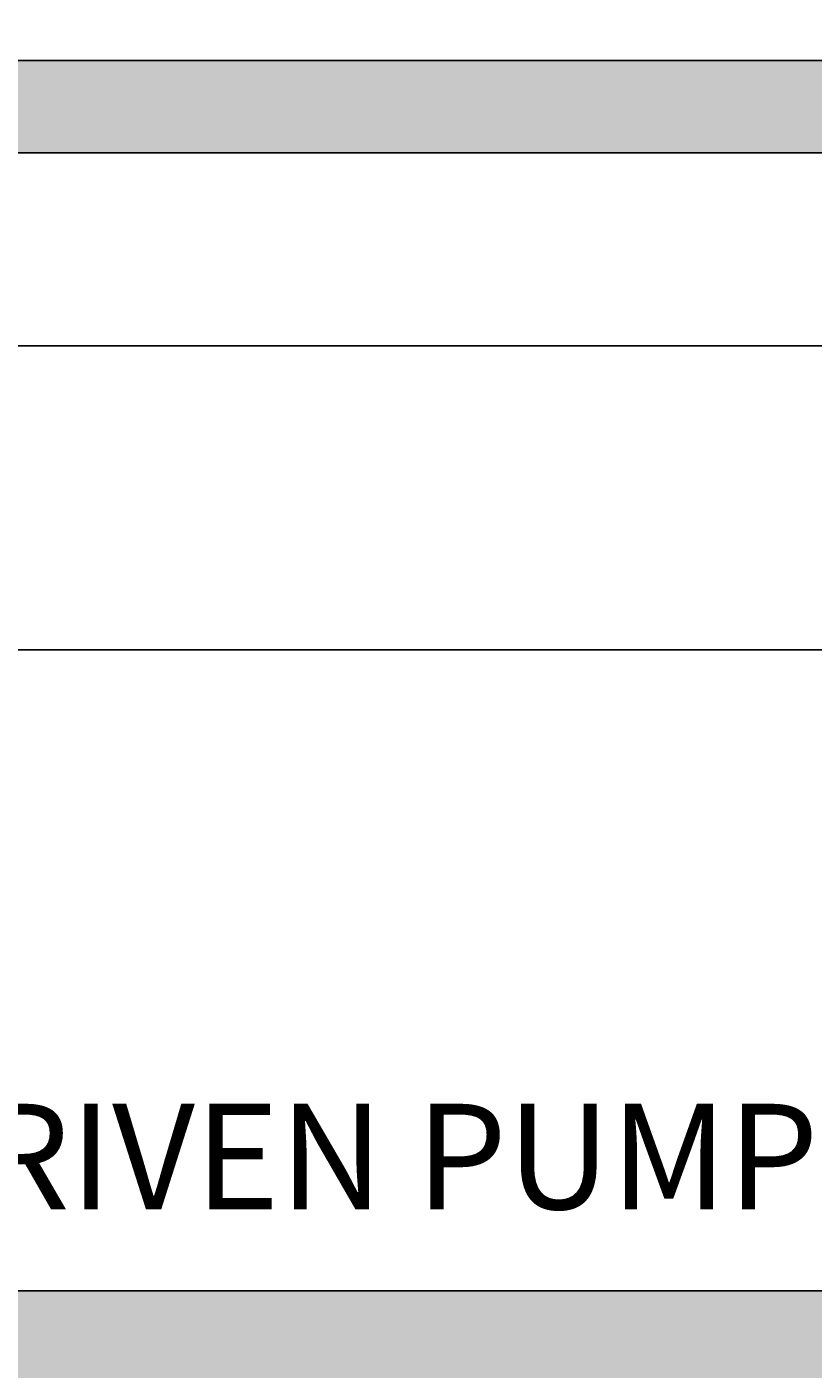
# Model space of a CAD drawing. Units: millimetres. Extents: x -11 to 280, y -4 to 208.
# Tile 43 of 55: x 121 to 151, y 106 to 157. Entities that reach past the tile are written whole.
import ezdxf

# ---------------------------------------------------------------- set-up
doc = ezdxf.new("R2010")
doc.units = ezdxf.units.MM
for name, color, linetype, lineweight in [('M-ANNO-TEXT', 7, 'Continuous', 18), ('M-DIMS', 2, 'Continuous', 18), ('M-HYDR-PRES', 7, 'Continuous', 25), ('M-HYDR-SUCT', 7, 'Continuous', 25)]:
    doc.layers.add(name, color=color, linetype=linetype, lineweight=lineweight)
doc.layers.add('M-HYDR-PRES-PATT', color=240, linetype='Continuous', lineweight=13, true_color=0xed1f24)
doc.layers.add('M-HYDR-SUCT-PATT', color=221, linetype='Continuous', lineweight=13, true_color=0xff7fdf)
doc.styles.get("Standard").update_dxf_attribs({"font": 'arial.ttf'})
doc.dimstyles.get("Standard").update_dxf_attribs({"dimtxt": 0.18, "dimasz": 0.18, "dimexe": 0.18, "dimexo": 0.0625, "dimgap": 0.09, "dimtad": 0, "dimtih": 1, "dimtoh": 1, "dimdec": 4, "dimzin": 0, "dimdsep": 46, "dimtxsty": 'Standard', "dimcen": 0.09, "dimadec": 0, "dimazin": 0, "dimtfac": 1, "dimtdec": 4, "dimtofl": 0, "dimtmove": 0, "dimatfit": 3, "dimfxl": 1, "dimtolj": 1, "dimtzin": 0, "dimarcsym": 0})

# ---------------------------------------------------------------- blocks, each defined once
blk = doc.blocks.new('*D5')
at = {"layer": 'Defpoints', "color": 0, "transparency": 16777216}
for p in [(24.759, 192.645), (-10.087, 11.435), (261.686, 11.435)]:
    blk.add_point(p, dxfattribs=at)
at = {"layer": 'M-DIMS', "color": 0, "lineweight": -2, "transparency": 16777216}
for p, q in [((24.696, 192.645), (-10.267, 192.645)), ((-10.087, 192.465), (-10.087, 102.222)), ((-10.087, 11.615), (-10.087, 101.858)), ((261.624, 11.435), (-10.267, 11.435))]:
    blk.add_line(p, q, dxfattribs=at)
at = {"layer": 'M-DIMS', "color": 0, "transparency": 16777216}
for points in [[(-10.117, 192.465), (-10.057, 192.465), (-10.087, 192.645)], [(-10.117, 11.615), (-10.057, 11.615), (-10.087, 11.435)]]:
    blk.add_solid(points, dxfattribs=at)
at = {"layer": 'M-DIMS', "color": 0, "transparency": 16777216, "insert": (-10.087, 102.04), "char_height": 0.18, "attachment_point": 5}
blk.add_mtext('\\A1;181.2', dxfattribs=at)
blk = doc.blocks.new('*D12')
at = {"layer": 'Defpoints', "color": 0, "transparency": 16777216}
for p in [(173.804, 207.495), (118.514, 96.485), (173.804, 89.387)]:
    blk.add_point(p, dxfattribs=at)
at = {"layer": 'M-DIMS', "color": 0, "lineweight": -2, "transparency": 16777216}
for p, q in [((118.514, 96.547), (118.514, 207.675)), ((118.694, 207.495), (145.765, 207.495)), ((173.624, 207.495), (146.553, 207.495)), ((173.804, 89.45), (173.804, 207.675))]:
    blk.add_line(p, q, dxfattribs=at)
at = {"layer": 'M-DIMS', "color": 0, "transparency": 16777216}
for points in [[(118.694, 207.525), (118.694, 207.465), (118.514, 207.495)], [(173.624, 207.525), (173.624, 207.465), (173.804, 207.495)]]:
    blk.add_solid(points, dxfattribs=at)
at = {"layer": 'M-DIMS', "color": 0, "transparency": 16777216, "insert": (146.159, 207.495), "char_height": 0.18, "attachment_point": 5}
blk.add_mtext('\\A1;55.29', dxfattribs=at)
blk = doc.blocks.new('*D14')
at = {"layer": 'Defpoints', "color": 0, "transparency": 16777216}
for p in [(-10.087, 144.661), (205.531, 144.661), (226.511, 133.123)]:
    blk.add_point(p, dxfattribs=at)
at = {"layer": 'M-DIMS', "color": 0, "lineweight": -2, "transparency": 16777216}
for p, q in [((205.469, 144.661), (-10.267, 144.661)), ((-10.087, 144.481), (-10.087, 139.074)), ((-10.087, 133.303), (-10.087, 138.71)), ((226.448, 133.123), (-10.267, 133.123))]:
    blk.add_line(p, q, dxfattribs=at)
at = {"layer": 'M-DIMS', "color": 0, "transparency": 16777216}
for points in [[(-10.117, 144.481), (-10.057, 144.481), (-10.087, 144.661)], [(-10.117, 133.303), (-10.057, 133.303), (-10.087, 133.123)]]:
    blk.add_solid(points, dxfattribs=at)
at = {"layer": 'M-DIMS', "color": 0, "transparency": 16777216, "insert": (-10.087, 138.892), "char_height": 0.18, "attachment_point": 5}
blk.add_mtext('\\A1;11.538', dxfattribs=at)

msp = doc.modelspace()

# ---------------------------------------------------------------- hatches: boundary and pattern name
at = {"layer": 'M-HYDR-PRES-PATT'}
h = msp.add_hatch(color=256, dxfattribs=at)
h.set_gradient(color1=(237, 31, 36), color2=(237, 31, 36), tint=1)
h.paths.add_polyline_path([(232.2, 133.1228), (228.7, 133.1228), (228.7, 108.8141), (102.7646, 108.8141), (102.7646, 105.3141), (232.2, 105.3141)])
h.paths.add_polyline_path([(128.8433, 105.3141), (125.3433, 105.3141), (125.3433, 91.7099, 1), (128.8433, 91.7099)])
h.paths.add_polyline_path([(229.1617, 78.7098), (196.7745, 78.7098, -0.4142136), (191.7745, 83.7098), (191.7745, 105.3141), (188.2745, 105.3141), (188.2745, 80.2098, 0.4142136), (193.2745, 75.2098), (225.6617, 75.2098), (225.6617, 43.5991), (229.1617, 43.5991)])
h.paths.add_polyline_path([(102.7646, 110.3704), (95.5776, 110.3704), (95.5776, 103.9022), (102.7646, 103.9022)])
h.paths.add_polyline_path([(100.7059, 107.2502), (99.1711, 106.3641), (99.1711, 106.8641), (97.1711, 106.8641), (97.1711, 107.6363), (99.1711, 107.6363), (99.1711, 108.1363)], flags=16)
h.paths.add_polyline_path([(234.6119, 138.4081), (226.5106, 138.4081), (226.5106, 133.1228), (234.6119, 133.1228)])
h.paths.add_polyline_path([(231.1963, 135.7055), (230.2965, 134.1786), (229.4241, 135.7213), (229.9241, 135.7168), (229.9418, 137.7167), (230.7141, 137.7099), (230.6963, 135.71)], flags=16)
at = {"layer": 'M-HYDR-SUCT-PATT'}
h = msp.add_hatch(color=256, dxfattribs=at)
h.set_gradient(color1=(255, 127, 223), color2=(255, 127, 223), tint=1, name='INVCYLINDER')
h.paths.add_polyline_path([(91.3629, 155.4768), (91.3629, 132.4768), (58.3629, 132.4768), (58.3629, 153.9768), (54.8629, 153.9768), (54.8629, 128.9768), (94.8629, 128.9768), (94.8629, 151.9768), (205.5315, 151.9768), (205.5315, 155.4768)])
h.paths.add_polyline_path([(91.3, 114.9452, 1), (78.8273, 114.9452), (78.8273, 108.8141), (42.6453, 108.8141), (42.6453, 153.9768), (39.1453, 153.9768), (39.1453, 105.3141), (78.8273, 105.3141), (78.8273, 98.1491, 1), (91.3, 98.1491), (91.3, 105.3141), (95.5776, 105.3141), (95.5776, 108.8141), (91.3, 108.8141)])
h.paths.add_polyline_path([(228.7, 138.4081), (232.2, 138.4081), (232.2, 144.6609), (228.7, 144.6609)])
h.paths.add_polyline_path([(253.1005, 151.9768, 1), (253.1005, 155.4768), (252.6001, 155.4768), (253.5249, 153.991, -0.1401047), (253.6005, 153.7268, -0.7542249), (252.676, 153.4626), (251.4221, 155.4768), (236.9353, 155.4768), (236.9353, 151.9768)])
h.paths.add_polyline_path([(30.8182, 40.7626), (30.8182, 36.7626), (60.8182, 36.7626), (60.8182, 40.7626)])

# ---------------------------------------------------------------- linework, layer by layer
at = {"layer": 'M-HYDR-PRES'}
msp.add_lwpolyline([(228.7, 133.1228), (228.7, 108.8141), (102.7646, 108.8141)], dxfattribs=at)
at = {"layer": 'M-HYDR-SUCT'}
for points in [[(58.3629, 153.9768), (58.3629, 132.4768), (91.3629, 132.4768), (91.3629, 155.4768), (205.5315, 155.4768)], [(54.8629, 153.9768), (54.8629, 128.9768), (94.8629, 128.9768), (94.8629, 151.9768), (205.5315, 151.9768)]]:
    msp.add_lwpolyline(points, dxfattribs=at)

# ---------------------------------------------------------------- texts
at = {"layer": 'M-ANNO-TEXT', "insert": (94.3856, 115.9056), "char_height": 4, "attachment_point": 1}
msp.add_mtext_dynamic_manual_height_columns('MOTOR-DRIVEN PUMP', width=63.617875, gutter_width=12.5, heights=[0], dxfattribs=at)

# ---------------------------------------------------------------- dimensions: what is measured, and where the dimension line sits
at = {"layer": 'M-DIMS'}
dim = msp.add_linear_dim(base=(173.8038, 207.495), p1=(118.5137, 96.4849), p2=(173.8038, 89.3873), dimstyle='Standard', override={"dimdec": 2, "dimlfac": 1, "dimrnd": 0, "dimzin": 0, "dimdsep": 46, "dimlunit": 2}, dxfattribs=at)
dim.commit()
dim.dimension.update_dxf_attribs({"geometry": '*D12', "text_midpoint": (146.1587, 207.495)})
for base, p1, p2, override, picture, middle in [((-10.0865, 11.4346), (24.7588, 192.645), (261.6863, 11.4346), {"dimdec": 1, "dimlfac": 1, "dimrnd": 0, "dimzin": 0, "dimdsep": 46, "dimlunit": 2}, '*D5', (-10.0865, 102.0398)), ((-10.0865, 144.6609), (226.5106, 133.1228), (205.5315, 144.6609), {"dimdec": 3, "dimlfac": 1, "dimrnd": 0, "dimzin": 0, "dimdsep": 46, "dimlunit": 2}, '*D14', (-10.0865, 138.8918))]:
    dim = msp.add_linear_dim(base=base, p1=p1, p2=p2, angle=90, dimstyle='Standard', override=override, dxfattribs=at)
    dim.commit()
    dim.dimension.update_dxf_attribs({"geometry": picture, "text_midpoint": middle})

doc.saveas('drawing.dxf')
